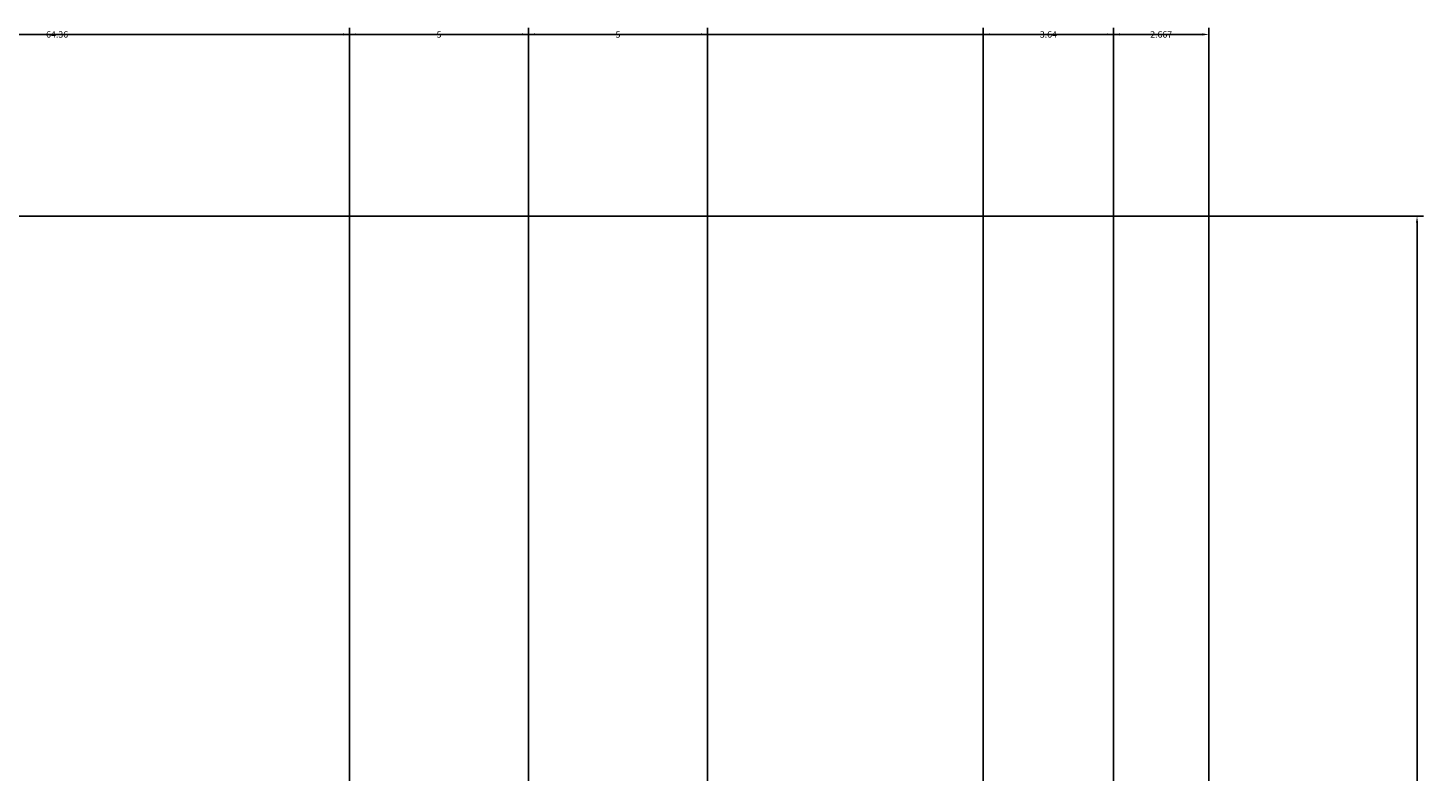
# Model space of a CAD drawing. Units: inches. Extents: x 237 to 313, y 343 to 451.
# Tile 6 of 6: x 274 to 313, y 430 to 451. Entities that reach past the tile are written whole.
import ezdxf

# ---------------------------------------------------------------- set-up
doc = ezdxf.new("R2010")
doc.units = ezdxf.units.IN
doc.header["$MEASUREMENT"] = 0
doc.layers.add('A-ANNO-DIMS', color=2, linetype='Continuous', lineweight=18)
doc.styles.get("Standard").update_dxf_attribs({"font": 'arial.ttf'})
doc.dimstyles.get("Standard").update_dxf_attribs({"dimtxt": 0.18, "dimasz": 0.18, "dimexe": 0.18, "dimexo": 0.0625, "dimgap": 0.09, "dimtad": 0, "dimtih": 1, "dimtoh": 1, "dimdec": 4, "dimzin": 0, "dimdsep": 46, "dimtxsty": 'Standard', "dimcen": 0.09, "dimadec": 0, "dimazin": 0, "dimtfac": 1, "dimtdec": 4, "dimtofl": 0, "dimtmove": 0, "dimatfit": 3, "dimfxl": 1, "dimtolj": 1, "dimtzin": 0, "dimarcsym": 0})

# ---------------------------------------------------------------- blocks, each defined once
blk = doc.blocks.new('*D3')
at = {"layer": 'A-ANNO-DIMS', "color": 0, "lineweight": -2, "transparency": 16777216}
for p, q in [((242.3, 363.785), (242.3, 451.078)), ((306.656, 382.738), (306.656, 451.078)), ((242.48, 450.898), (274.084, 450.898)), ((306.476, 450.898), (274.872, 450.898))]:
    blk.add_line(p, q, dxfattribs=at)
at = {"layer": 'A-ANNO-DIMS', "color": 0, "lineweight": 35, "transparency": 16777216}
for points in [[(242.48, 450.928), (242.48, 450.868), (242.3, 450.898)], [(306.476, 450.928), (306.476, 450.868), (306.656, 450.898)]]:
    blk.add_solid(points, dxfattribs=at)
at = {"layer": 'Defpoints', "color": 0, "lineweight": 35, "transparency": 16777216}
for p in [(306.656, 450.898), (306.656, 382.675), (242.3, 363.723)]:
    blk.add_point(p, dxfattribs=at)
at = {"layer": 'A-ANNO-DIMS', "color": 0, "transparency": 16777216, "insert": (274.478, 450.898), "char_height": 0.18, "attachment_point": 5}
blk.add_mtext('\\A1;64.36', dxfattribs=at)
blk = doc.blocks.new('*D4')
at = {"layer": 'A-ANNO-DIMS', "color": 0, "lineweight": -2, "transparency": 16777216}
for p, q in [((258.115, 445.823), (312.65, 445.823)), ((312.47, 445.643), (312.47, 397.21)), ((312.47, 348.414), (312.47, 396.846)), ((289.124, 348.234), (312.65, 348.234))]:
    blk.add_line(p, q, dxfattribs=at)
at = {"layer": 'A-ANNO-DIMS', "color": 0, "lineweight": 35, "transparency": 16777216}
for points in [[(312.44, 445.643), (312.5, 445.643), (312.47, 445.823)], [(312.44, 348.414), (312.5, 348.414), (312.47, 348.234)]]:
    blk.add_solid(points, dxfattribs=at)
at = {"layer": 'Defpoints', "color": 0, "lineweight": 35, "transparency": 16777216}
for p in [(258.052, 445.823), (289.062, 348.234), (312.47, 348.234)]:
    blk.add_point(p, dxfattribs=at)
at = {"layer": 'A-ANNO-DIMS', "color": 0, "transparency": 16777216, "insert": (312.47, 397.028), "char_height": 0.18, "attachment_point": 5}
blk.add_mtext('\\A1;97.59', dxfattribs=at)
blk = doc.blocks.new('*D7')
at = {"layer": 'A-ANNO-DIMS', "color": 0, "lineweight": -2, "transparency": 16777216}
for p, q in [((257.997, 436.662), (257.997, 451.078)), ((282.648, 418.461), (282.648, 451.078)), ((258.177, 450.898), (269.926, 450.898)), ((282.468, 450.898), (270.718, 450.898))]:
    blk.add_line(p, q, dxfattribs=at)
at = {"layer": 'A-ANNO-DIMS', "color": 0, "lineweight": 35, "transparency": 16777216}
for points in [[(258.177, 450.928), (258.177, 450.868), (257.997, 450.898)], [(282.468, 450.928), (282.468, 450.868), (282.648, 450.898)]]:
    blk.add_solid(points, dxfattribs=at)
at = {"layer": 'Defpoints', "color": 0, "lineweight": 35, "transparency": 16777216}
for p in [(282.648, 450.898), (257.997, 436.599), (282.648, 418.399)]:
    blk.add_point(p, dxfattribs=at)
at = {"layer": 'A-ANNO-DIMS', "color": 0, "transparency": 16777216, "insert": (270.322, 450.898), "char_height": 0.18, "attachment_point": 5}
blk.add_mtext('\\A1;24.65', dxfattribs=at)
blk = doc.blocks.new('*D8')
at = {"layer": 'A-ANNO-DIMS', "color": 0, "lineweight": -2, "transparency": 16777216}
for p, q in [((282.648, 418.461), (282.648, 451.078)), ((287.648, 422.133), (287.648, 451.078)), ((282.828, 450.898), (284.998, 450.898)), ((287.468, 450.898), (285.297, 450.898))]:
    blk.add_line(p, q, dxfattribs=at)
at = {"layer": 'A-ANNO-DIMS', "color": 0, "lineweight": 35, "transparency": 16777216}
for points in [[(282.828, 450.928), (282.828, 450.868), (282.648, 450.898)], [(287.468, 450.928), (287.468, 450.868), (287.648, 450.898)]]:
    blk.add_solid(points, dxfattribs=at)
at = {"layer": 'Defpoints', "color": 0, "lineweight": 35, "transparency": 16777216}
for p in [(287.648, 450.898), (287.648, 422.07), (282.648, 418.399)]:
    blk.add_point(p, dxfattribs=at)
at = {"layer": 'A-ANNO-DIMS', "color": 0, "transparency": 16777216, "insert": (285.148, 450.898), "char_height": 0.18, "attachment_point": 5}
blk.add_mtext('\\A1;5', dxfattribs=at)
blk = doc.blocks.new('*D9')
at = {"layer": 'A-ANNO-DIMS', "color": 0, "lineweight": -2, "transparency": 16777216}
for p, q in [((287.648, 422.133), (287.648, 451.078)), ((292.648, 428.708), (292.648, 451.078)), ((287.828, 450.898), (289.998, 450.898)), ((292.468, 450.898), (290.297, 450.898))]:
    blk.add_line(p, q, dxfattribs=at)
at = {"layer": 'A-ANNO-DIMS', "color": 0, "lineweight": 35, "transparency": 16777216}
for points in [[(287.828, 450.928), (287.828, 450.868), (287.648, 450.898)], [(292.468, 450.928), (292.468, 450.868), (292.648, 450.898)]]:
    blk.add_solid(points, dxfattribs=at)
at = {"layer": 'Defpoints', "color": 0, "lineweight": 35, "transparency": 16777216}
for p in [(292.648, 450.898), (292.648, 428.646), (287.648, 422.07)]:
    blk.add_point(p, dxfattribs=at)
at = {"layer": 'A-ANNO-DIMS', "color": 0, "transparency": 16777216, "insert": (290.148, 450.898), "char_height": 0.18, "attachment_point": 5}
blk.add_mtext('\\A1;5', dxfattribs=at)
blk = doc.blocks.new('*D10')
at = {"layer": 'A-ANNO-DIMS', "color": 0, "lineweight": -2, "transparency": 16777216}
for p, q in [((300.353, 382.738), (300.353, 451.078)), ((303.989, 382.738), (303.989, 451.078)), ((300.533, 450.898), (301.848, 450.898)), ((303.809, 450.898), (302.495, 450.898))]:
    blk.add_line(p, q, dxfattribs=at)
at = {"layer": 'A-ANNO-DIMS', "color": 0, "lineweight": 35, "transparency": 16777216}
for points in [[(300.533, 450.928), (300.533, 450.868), (300.353, 450.898)], [(303.809, 450.928), (303.809, 450.868), (303.989, 450.898)]]:
    blk.add_solid(points, dxfattribs=at)
at = {"layer": 'Defpoints', "color": 0, "lineweight": 35, "transparency": 16777216}
for p in [(303.989, 450.898), (300.353, 382.675), (303.989, 382.675)]:
    blk.add_point(p, dxfattribs=at)
at = {"layer": 'A-ANNO-DIMS', "color": 0, "transparency": 16777216, "insert": (302.171, 450.898), "char_height": 0.18, "attachment_point": 5}
blk.add_mtext('\\A1;3.64', dxfattribs=at)
blk = doc.blocks.new('*D11')
at = {"layer": 'A-ANNO-DIMS', "color": 0, "lineweight": -2, "transparency": 16777216}
for p, q in [((303.989, 382.738), (303.989, 451.078)), ((306.656, 382.738), (306.656, 451.078)), ((304.169, 450.898), (304.928, 450.898)), ((306.476, 450.898), (305.718, 450.898))]:
    blk.add_line(p, q, dxfattribs=at)
at = {"layer": 'A-ANNO-DIMS', "color": 0, "lineweight": 35, "transparency": 16777216}
for points in [[(304.169, 450.928), (304.169, 450.868), (303.989, 450.898)], [(306.476, 450.928), (306.476, 450.868), (306.656, 450.898)]]:
    blk.add_solid(points, dxfattribs=at)
at = {"layer": 'Defpoints', "color": 0, "lineweight": 35, "transparency": 16777216}
for p in [(306.656, 450.898), (303.989, 382.675), (306.656, 382.675)]:
    blk.add_point(p, dxfattribs=at)
at = {"layer": 'A-ANNO-DIMS', "color": 0, "transparency": 16777216, "insert": (305.323, 450.898), "char_height": 0.18, "attachment_point": 5}
blk.add_mtext('\\A1;2.667', dxfattribs=at)

msp = doc.modelspace()

# ---------------------------------------------------------------- dimensions: what is measured, and where the dimension line sits
at = {"layer": 'A-ANNO-DIMS'}
for base, p1, p2, override, picture, middle in [((306.6564, 450.8976), (242.3002, 363.7227), (306.6564, 382.675), {"dimdec": 2, "dimlfac": 1, "dimrnd": 0, "dimzin": 0, "dimdsep": 46, "dimlunit": 2}, '*D3', (274.4783, 450.8976)), ((282.6477, 450.8976), (257.9968, 436.5992), (282.6477, 418.3988), {"dimdec": 2, "dimlfac": 1, "dimrnd": 0, "dimzin": 0, "dimdsep": 46, "dimlunit": 2}, '*D7', (270.3223, 450.8976)), ((287.6477, 450.8976), (282.6477, 418.3988), (287.6477, 422.0704), {"dimdec": 0, "dimlfac": 1, "dimrnd": 0, "dimzin": 0, "dimdsep": 46, "dimlunit": 2}, '*D8', (285.1477, 450.8976)), ((292.6477, 450.8976), (287.6477, 422.0704), (292.6477, 428.6459), {"dimdec": 0, "dimlfac": 1, "dimrnd": 0, "dimzin": 0, "dimdsep": 46, "dimlunit": 2}, '*D9', (290.1477, 450.8976)), ((303.9895, 450.8976), (300.3529, 382.675), (303.9895, 382.675), {"dimdec": 2, "dimlfac": 1, "dimrnd": 0, "dimzin": 0, "dimdsep": 46, "dimlunit": 2}, '*D10', (302.1712, 450.8976)), ((306.6564, 450.8976), (303.9895, 382.675), (306.6564, 382.675), {"dimdec": 3, "dimlfac": 1, "dimrnd": 0, "dimzin": 0, "dimdsep": 46, "dimlunit": 2}, '*D11', (305.3229, 450.8976))]:
    dim = msp.add_linear_dim(base=base, p1=p1, p2=p2, dimstyle='Standard', override=override, dxfattribs=at)
    dim.commit()
    dim.dimension.update_dxf_attribs({"geometry": picture, "text_midpoint": middle})
dim = msp.add_linear_dim(base=(312.4701, 348.2337), p1=(258.0525, 445.8226), p2=(289.0615, 348.2337), angle=90, dimstyle='Standard', override={"dimdec": 2, "dimlfac": 1, "dimrnd": 0, "dimzin": 0, "dimdsep": 46, "dimlunit": 2}, dxfattribs=at)
dim.commit()
dim.dimension.update_dxf_attribs({"geometry": '*D4', "text_midpoint": (312.4701, 397.0282)})

doc.saveas('drawing.dxf')
